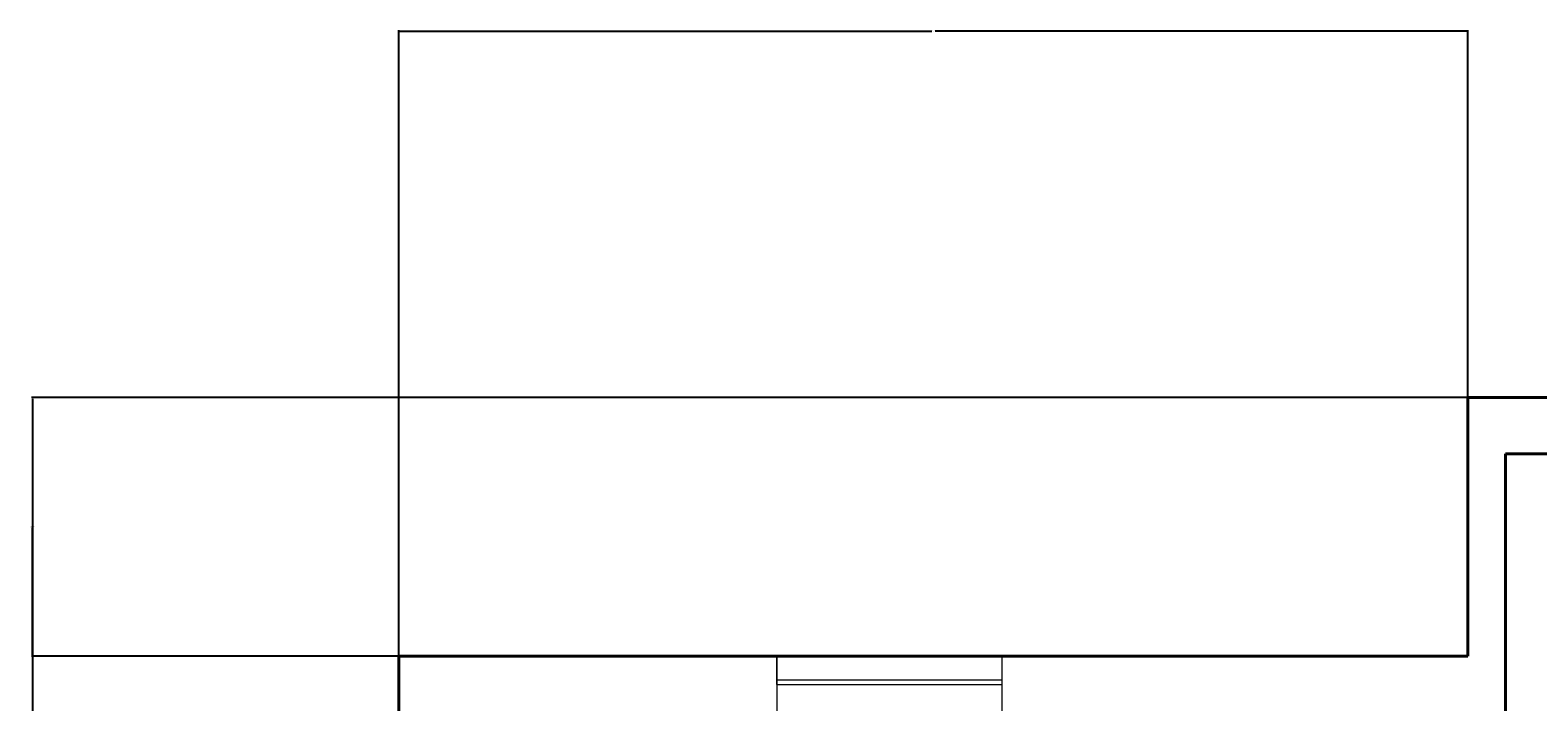
# Model space of a CAD drawing. Units: inches. Extents: x -46 to 1145, y -527 to 760.
# Tile 44 of 57: x -46 to 195, y 652 to 760. Entities that reach past the tile are written whole.
import ezdxf

# ---------------------------------------------------------------- set-up
doc = ezdxf.new("R2010")
doc.units = ezdxf.units.IN
doc.header["$MEASUREMENT"] = 0
for name, color, linetype, lineweight in [('A-ANNO-DIMS', 2, 'Continuous', 18), ('WALLS', 4, 'Continuous', 40), ('WINDOWS', 240, 'Continuous', 20)]:
    doc.layers.add(name, color=color, linetype=linetype, lineweight=lineweight)
doc.styles.get("Standard").update_dxf_attribs({"font": 'arial.ttf'})
doc.dimstyles.get("Standard").update_dxf_attribs({"dimtxt": 0.18, "dimasz": 0.18, "dimexe": 0.18, "dimexo": 0.0625, "dimgap": 0.09, "dimtad": 0, "dimtih": 1, "dimtoh": 1, "dimdec": 0, "dimzin": 0, "dimdsep": 46, "dimlunit": 3, "dimtxsty": 'Standard', "dimcen": 0.09, "dimadec": 0, "dimazin": 0, "dimtfac": 1, "dimtdec": 0, "dimtofl": 0, "dimtmove": 0, "dimatfit": 3, "dimfxl": 1, "dimtolj": 1, "dimtzin": 0, "dimarcsym": 0})

# ---------------------------------------------------------------- blocks, each defined once
blk = doc.blocks.new('WINDOW-36IN')
for p, q in [((0, 4.5), (0, 9)), ((0, 9), (0, 0)), ((36, 9), (36, 0)), ((0, 5.23), (36, 5.23)), ((0, 4.5), (36, 4.5))]:
    blk.add_line(p, q)
blk = doc.blocks.new('*D685')
at = {"layer": 'A-ANNO-DIMS', "color": 0, "lineweight": -2, "transparency": 16777216}
for p, q in [((183.5, 700.89), (-46.22, 700.89)), ((-46.04, 700.71), (-46.04, 116.39)), ((-46.04, -468.3), (-46.04, 116.02)), ((12.5, -468.48), (-46.22, -468.48))]:
    blk.add_line(p, q, dxfattribs=at)
at = {"layer": 'A-ANNO-DIMS', "color": 0, "transparency": 16777216}
for points in [[(-46.07, 700.71), (-46.01, 700.71), (-46.04, 700.89)], [(-46.07, -468.3), (-46.01, -468.3), (-46.04, -468.48)]]:
    blk.add_solid(points, dxfattribs=at)
at = {"layer": 'Defpoints', "color": 0, "transparency": 16777216}
for p in [(-46.04, 700.89), (183.56, 700.89), (12.56, -468.48)]:
    blk.add_point(p, dxfattribs=at)
at = {"layer": 'A-ANNO-DIMS', "color": 0, "transparency": 16777216, "insert": (-46.04, 116.2), "char_height": 0.18, "attachment_point": 5}
blk.add_mtext('\\A1;1169.4', dxfattribs=at)
blk = doc.blocks.new('*D690')
at = {"layer": 'A-ANNO-DIMS', "color": 0, "lineweight": -2, "transparency": 16777216}
for p, q in [((183.5, 700.89), (-46.22, 700.89)), ((-46.04, 700.71), (-46.04, 680.39)), ((-46.04, 659.7), (-46.04, 680.02)), ((183.5, 659.52), (-46.22, 659.52))]:
    blk.add_line(p, q, dxfattribs=at)
at = {"layer": 'A-ANNO-DIMS', "color": 0, "transparency": 16777216}
for points in [[(-46.07, 700.71), (-46.01, 700.71), (-46.04, 700.89)], [(-46.07, 659.7), (-46.01, 659.7), (-46.04, 659.52)]]:
    blk.add_solid(points, dxfattribs=at)
at = {"layer": 'Defpoints', "color": 0, "transparency": 16777216}
for p in [(-46.04, 700.89), (183.56, 700.89), (183.56, 659.52)]:
    blk.add_point(p, dxfattribs=at)
at = {"layer": 'A-ANNO-DIMS', "color": 0, "transparency": 16777216, "insert": (-46.04, 680.2), "char_height": 0.18, "attachment_point": 5}
blk.add_mtext('\\A1;41.37', dxfattribs=at)
blk = doc.blocks.new('*D697')
at = {"layer": 'A-ANNO-DIMS', "color": 0, "lineweight": -2, "transparency": 16777216}
for p, q in [((12.56, 659.58), (12.56, 759.67)), ((183.56, 659.58), (183.56, 759.67)), ((12.74, 759.49), (97.8, 759.49)), ((183.38, 759.49), (98.33, 759.49))]:
    blk.add_line(p, q, dxfattribs=at)
at = {"layer": 'A-ANNO-DIMS', "color": 0, "transparency": 16777216}
for points in [[(12.74, 759.52), (12.74, 759.46), (12.56, 759.49)], [(183.38, 759.52), (183.38, 759.46), (183.56, 759.49)]]:
    blk.add_solid(points, dxfattribs=at)
at = {"layer": 'Defpoints', "color": 0, "transparency": 16777216}
for p in [(183.56, 759.49), (12.56, 659.52), (183.56, 659.52)]:
    blk.add_point(p, dxfattribs=at)
at = {"layer": 'A-ANNO-DIMS', "color": 0, "transparency": 16777216, "insert": (98.06, 759.49), "char_height": 0.18, "attachment_point": 5}
blk.add_mtext('\\A1;171', dxfattribs=at)

msp = doc.modelspace()

# ---------------------------------------------------------------- linework, layer by layer
at = {"layer": 'WALLS'}
for p, q in [((183.5637, 659.5176), (183.5637, 700.8886)), ((183.5637, 700.8886), (189.5637, 700.8886)), ((189.5637, 700.8886), (339.5637, 700.8886)), ((189.5637, 691.8886), (333.5637, 691.8886)), ((189.5637, 659.5176), (189.5637, 691.8886)), ((12.5637, 659.5176), (12.5637, 221.5176)), ((12.5637, 659.5176), (183.5637, 659.5176)), ((189.5637, 659.5176), (189.5637, 500.5176))]:
    msp.add_line(p, q, dxfattribs=at)

# ---------------------------------------------------------------- block references
at = {"layer": 'WINDOWS'}
msp.add_blockref('WINDOW-36IN', (72.995, 650.518), dxfattribs=at)

# ---------------------------------------------------------------- dimensions: what is measured, and where the dimension line sits
at = {"layer": 'A-ANNO-DIMS'}
dim = msp.add_linear_dim(base=(183.5637, 759.4886), p1=(12.5637, 659.5176), p2=(183.5637, 659.5176), dimstyle='Standard', override={"dimdec": 0, "dimlfac": 1, "dimrnd": 0, "dimzin": 0, "dimdsep": 46, "dimlunit": 2}, dxfattribs=at)
dim.commit()
dim.dimension.update_dxf_attribs({"geometry": '*D697', "text_midpoint": (98.0637, 759.4886)})
for p1, override, picture, middle in [((12.5637, -468.4824), {"dimdec": 1, "dimlfac": 1, "dimrnd": 0, "dimzin": 0, "dimdsep": 46, "dimlunit": 2}, '*D685', (-46.0363, 116.2031)), ((183.5637, 659.5176), {"dimdec": 2, "dimlfac": 1, "dimrnd": 0, "dimzin": 0, "dimdsep": 46, "dimlunit": 2}, '*D690', (-46.0363, 680.2031))]:
    dim = msp.add_linear_dim(base=(-46.0363, 700.8886), p1=p1, p2=(183.5637, 700.8886), angle=90, dimstyle='Standard', override=override, dxfattribs=at)
    dim.commit()
    dim.dimension.update_dxf_attribs({"geometry": picture, "text_midpoint": middle})

doc.saveas('drawing.dxf')
